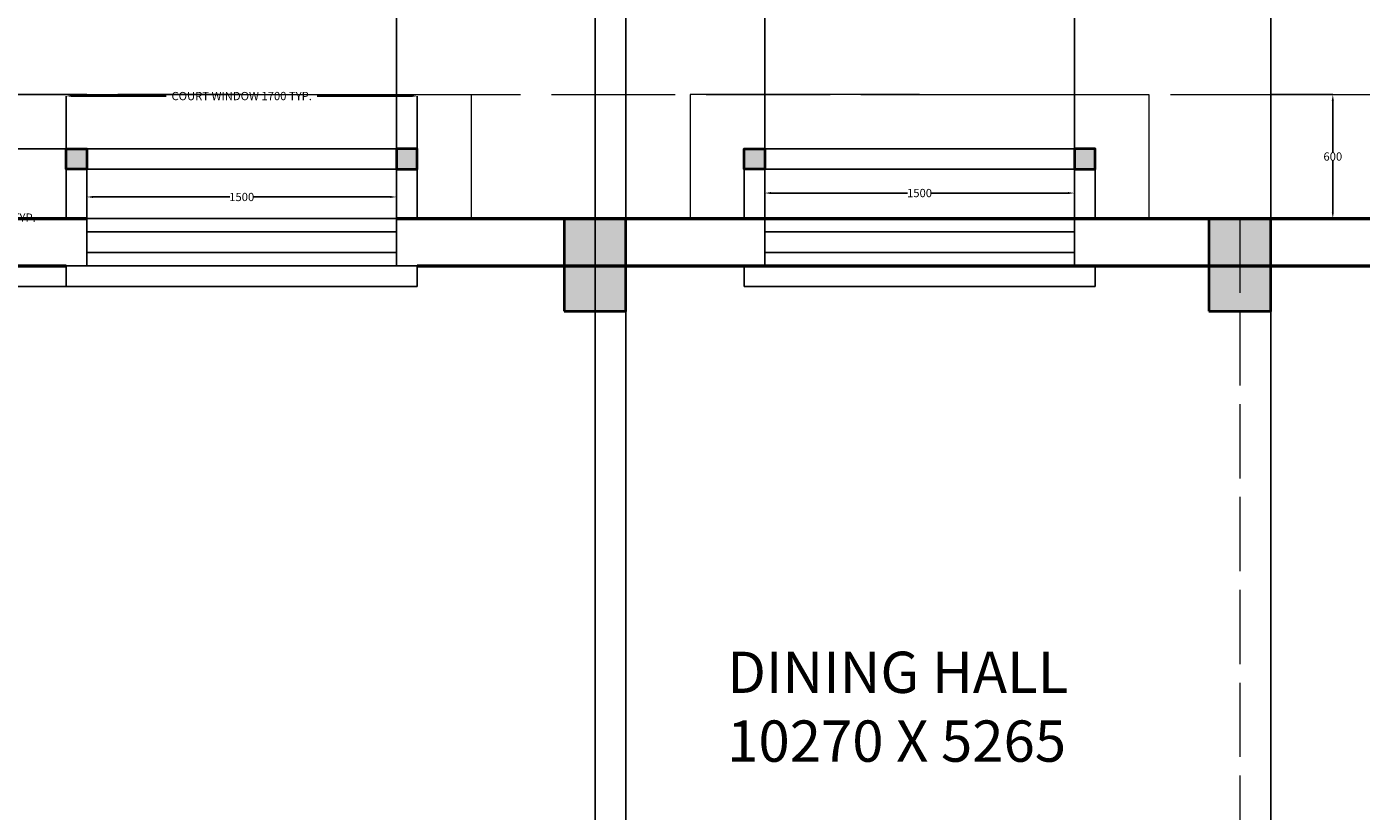
# Model space of a CAD drawing. Units: millimetres. Extents: x -17156 to 39375, y -45872 to -24892.
# Tile 7 of 12: x -5337 to 1128, y -37711 to -33909. Entities that reach past the tile are written whole.
import ezdxf

# ---------------------------------------------------------------- set-up
doc = ezdxf.new("R2010")
doc.units = ezdxf.units.MM
doc.header["$MEASUREMENT"] = 0
doc.linetypes.add('ACAD_ISO02W100', pattern=[15, 12, -3])
for name, color, linetype, lineweight in [('A-ANNO-DIMS', 2, 'Continuous', 18), ('A-AREA-IDEN', 4, 'Continuous', 25), ('A-COLS', 7, 'Continuous', 40), ('A-ROOF', 8, 'Continuous', 18), ('A-ROOF-OVHD', 8, 'ACAD_ISO02W100', 18), ('S-BEAM-OVHD', 8, 'ACAD_ISO02W100', 18), ('WALLS', 5, 'Continuous', 50), ('WINDOW', 240, 'Continuous', 25)]:
    doc.layers.add(name, color=color, linetype=linetype, lineweight=lineweight)
doc.layers.add('A-COLS-PATT', color=114, linetype='Continuous', lineweight=13, true_color=0x139b48)
doc.styles.get("Standard").update_dxf_attribs({"font": 'arial.ttf'})
doc.dimstyles.get("Standard").update_dxf_attribs({"dimtxt": 40, "dimasz": 30.18, "dimexe": 0, "dimexo": 0.0625, "dimgap": 0.09, "dimtad": 0, "dimtih": 1, "dimtoh": 1, "dimdec": 0, "dimzin": 0, "dimdsep": 46, "dimtxsty": 'Standard', "dimcen": 0.09, "dimadec": 0, "dimazin": 0, "dimtfac": 1, "dimtdec": 0, "dimtofl": 0, "dimtmove": 0, "dimatfit": 3, "dimfxl": 1, "dimtolj": 1, "dimtzin": 0, "dimarcsym": 0})

# ---------------------------------------------------------------- blocks, each defined once
blk = doc.blocks.new('*D100')
at = {"layer": 'A-ANNO-DIMS', "color": 0, "lineweight": -2, "transparency": 16777216}
for p, q in [((-5045.8, -34837.8), (-5045.8, -34733.9)), ((-5015.7, -34733.9), (-4353.7, -34733.9)), ((-3576, -34733.9), (-4238, -34733.9)), ((-3545.8, -34837.8), (-3545.8, -34733.9))]:
    blk.add_line(p, q, dxfattribs=at)
at = {"layer": 'A-ANNO-DIMS', "color": 0, "lineweight": 100, "transparency": 16777216}
for points in [[(-5015.7, -34728.9), (-5015.7, -34738.9), (-5045.8, -34733.9)], [(-3576, -34728.9), (-3576, -34738.9), (-3545.8, -34733.9)]]:
    blk.add_solid(points, dxfattribs=at)
at = {"layer": 'Defpoints', "color": 0, "lineweight": 100, "transparency": 16777216}
for p in [(-3545.8, -34733.9), (-5045.8, -34837.8), (-3545.8, -34837.8)]:
    blk.add_point(p, dxfattribs=at)
at = {"layer": 'A-ANNO-DIMS', "color": 0, "transparency": 16777216, "insert": (-4295.8, -34733.9), "char_height": 40, "attachment_point": 5}
blk.add_mtext('\\A1;1500', dxfattribs=at)
blk = doc.blocks.new('*D101')
at = {"layer": 'A-ANNO-DIMS', "color": 0, "lineweight": -2, "transparency": 16777216}
for p, q in [((-1762.3, -34837.8), (-1762.3, -34714.9)), ((-1732.1, -34714.9), (-1070.2, -34714.9)), ((-292.5, -34714.9), (-954.4, -34714.9)), ((-262.3, -34837.8), (-262.3, -34714.9))]:
    blk.add_line(p, q, dxfattribs=at)
at = {"layer": 'A-ANNO-DIMS', "color": 0, "lineweight": 100, "transparency": 16777216}
for points in [[(-1732.1, -34709.8), (-1732.1, -34719.9), (-1762.3, -34714.9)], [(-292.5, -34709.8), (-292.5, -34719.9), (-262.3, -34714.9)]]:
    blk.add_solid(points, dxfattribs=at)
at = {"layer": 'Defpoints', "color": 0, "lineweight": 100, "transparency": 16777216}
for p in [(-262.3, -34714.9), (-1762.3, -34837.8), (-262.3, -34837.8)]:
    blk.add_point(p, dxfattribs=at)
at = {"layer": 'A-ANNO-DIMS', "color": 0, "transparency": 16777216, "insert": (-1012.3, -34714.9), "char_height": 40, "attachment_point": 5}
blk.add_mtext('\\A1;1500', dxfattribs=at)
blk = doc.blocks.new('*D112')
at = {"layer": 'A-ANNO-DIMS', "color": 0, "lineweight": -2, "transparency": 16777216}
for p, q in [((686.4, -34237.8), (989.7, -34237.8)), ((989.7, -34268), (989.7, -34517.3)), ((989.7, -34807.7), (989.7, -34558.4)), ((689.7, -34837.8), (989.7, -34837.8))]:
    blk.add_line(p, q, dxfattribs=at)
at = {"layer": 'A-ANNO-DIMS', "color": 0, "lineweight": 100, "transparency": 16777216}
for points in [[(984.6, -34268), (994.7, -34268), (989.7, -34237.8)], [(984.6, -34807.7), (994.7, -34807.7), (989.7, -34837.8)]]:
    blk.add_solid(points, dxfattribs=at)
at = {"layer": 'Defpoints', "color": 0, "lineweight": 100, "transparency": 16777216}
for p in [(686.3, -34237.8), (689.7, -34837.8), (989.7, -34837.8)]:
    blk.add_point(p, dxfattribs=at)
at = {"layer": 'A-ANNO-DIMS', "color": 0, "transparency": 16777216, "insert": (989.7, -34537.8), "char_height": 40, "attachment_point": 5}
blk.add_mtext('\\A1;600', dxfattribs=at)
blk = doc.blocks.new('WIN-COURTYARD-1500')
for p, q in [((1600, 668), (100, 668)), ((0, 568), (0, 330)), ((100, 568), (100, 330)), ((1600, 568), (100, 568)), ((1600, 568), (1600, 330)), ((1700, 568), (1700, 330)), ((100, 330), (100, 100)), ((100, 330), (1600, 330)), ((1600, 330), (1600, 100)), ((100, 265), (1600, 265)), ((100, 165), (1600, 165)), ((0, 100), (0, 0)), ((0, 100), (100, 100)), ((100, 100), (1700, 100)), ((1700, 0), (1700, 100)), ((0, 0), (1700, 0))]:
    blk.add_line(p, q)
blk = doc.blocks.new('COL-450x300')
h = blk.add_hatch(color=256)
h.dxf.hatch_style = 1
h.paths.add_polyline_path([(0, 300), (0, 0), (450, 0), (450, 300)])
blk.add_lwpolyline([(0, 300), (0, 0), (450, 0), (450, 300)], close=True)
blk = doc.blocks.new('WINDOW-HOOD-2223x600')
for p, q in [((0, 600), (0, 0)), ((1111.5, 600), (0, 600)), ((1111.5, 600), (2223, 600)), ((2223, 600), (2223, 0))]:
    blk.add_line(p, q)
blk = doc.blocks.new('*D140')
at = {"layer": 'A-ANNO-DIMS', "color": 0, "lineweight": -2, "transparency": 16777216}
for p, q in [((-5145.8, -34499.8), (-5145.8, -34244.8)), ((-5115.7, -34244.8), (-4661.6, -34244.8)), ((-3476, -34244.8), (-3930.1, -34244.8)), ((-3445.8, -34499.8), (-3445.8, -34244.8))]:
    blk.add_line(p, q, dxfattribs=at)
at = {"layer": 'A-ANNO-DIMS', "color": 0, "lineweight": 100, "transparency": 16777216}
for points in [[(-5115.7, -34239.8), (-5115.7, -34249.9), (-5145.8, -34244.8)], [(-3476, -34239.8), (-3476, -34249.9), (-3445.8, -34244.8)]]:
    blk.add_solid(points, dxfattribs=at)
at = {"layer": 'Defpoints', "color": 0, "lineweight": 100, "transparency": 16777216}
for p in [(-3445.8, -34244.8), (-5145.8, -34499.8), (-3445.8, -34499.8)]:
    blk.add_point(p, dxfattribs=at)
at = {"layer": 'A-ANNO-DIMS', "color": 0, "transparency": 16777216, "insert": (-4295.8, -34244.8), "char_height": 40, "attachment_point": 5}
blk.add_mtext('\\A1;COURT WINDOW 1700 TYP.', dxfattribs=at)
blk = doc.blocks.new('*D141')
at = {"layer": 'A-ANNO-DIMS', "color": 0, "lineweight": -2, "transparency": 16777216}
for p, q in [((-5145.9, -34499.8), (-5400.8, -34499.8)), ((-5400.8, -34530), (-5400.8, -34813.3)), ((-5400.8, -35137.7), (-5400.8, -34854.4)), ((-5145.9, -35167.8), (-5400.8, -35167.8))]:
    blk.add_line(p, q, dxfattribs=at)
at = {"layer": 'A-ANNO-DIMS', "color": 0, "lineweight": 100, "transparency": 16777216}
for points in [[(-5405.9, -34530), (-5395.8, -34530), (-5400.8, -34499.8)], [(-5405.9, -35137.7), (-5395.8, -35137.7), (-5400.8, -35167.8)]]:
    blk.add_solid(points, dxfattribs=at)
at = {"layer": 'Defpoints', "color": 0, "lineweight": 100, "transparency": 16777216}
for p in [(-5400.8, -34499.8), (-5145.8, -34499.8), (-5145.8, -35167.8)]:
    blk.add_point(p, dxfattribs=at)
at = {"layer": 'A-ANNO-DIMS', "color": 0, "transparency": 16777216, "insert": (-5400.8, -34833.8), "char_height": 40, "attachment_point": 5}
blk.add_mtext('\\A1;668 TYP.', dxfattribs=at)
blk = doc.blocks.new('*D145')
at = {"layer": 'A-ANNO-DIMS', "color": 0, "lineweight": -2, "transparency": 16777216}
for p, q in [((-6237.4, -27247.8), (-17080.3, -27247.8)), ((-17080.3, -27278), (-17080.3, -35684.8)), ((-17080.3, -44132.7), (-17080.3, -35725.9)), ((-2887.4, -44162.8), (-17080.3, -44162.8))]:
    blk.add_line(p, q, dxfattribs=at)
at = {"layer": 'A-ANNO-DIMS', "color": 0, "lineweight": 100, "transparency": 16777216}
for points in [[(-17085.4, -27278), (-17075.3, -27278), (-17080.3, -27247.8)], [(-17085.4, -44132.7), (-17075.3, -44132.7), (-17080.3, -44162.8)]]:
    blk.add_solid(points, dxfattribs=at)
at = {"layer": 'Defpoints', "color": 0, "lineweight": 100, "transparency": 16777216}
for p in [(-6237.3, -27247.8), (-17080.3, -44162.8), (-2887.3, -44162.8)]:
    blk.add_point(p, dxfattribs=at)
at = {"layer": 'A-ANNO-DIMS', "color": 0, "transparency": 16777216, "insert": (-17080.3, -35705.3), "char_height": 40, "attachment_point": 5}
blk.add_mtext('\\A1;16915', dxfattribs=at)
blk = doc.blocks.new('*D148')
at = {"layer": 'A-ANNO-DIMS', "color": 0, "lineweight": -2, "transparency": 16777216}
for p, q in [((-3545.8, -34837.8), (-3545.8, -25564.8)), ((-3515.7, -25564.8), (-2735.5, -25564.8)), ((-1792.5, -25564.8), (-2572.7, -25564.8)), ((-1762.3, -34837.8), (-1762.3, -25564.8))]:
    blk.add_line(p, q, dxfattribs=at)
at = {"layer": 'A-ANNO-DIMS', "color": 0, "lineweight": 100, "transparency": 16777216}
for points in [[(-3515.7, -25559.8), (-3515.7, -25569.9), (-3545.8, -25564.8)], [(-1792.5, -25559.8), (-1792.5, -25569.9), (-1762.3, -25564.8)]]:
    blk.add_solid(points, dxfattribs=at)
at = {"layer": 'Defpoints', "color": 0, "lineweight": 100, "transparency": 16777216}
for p in [(-1762.3, -25564.8), (-3545.8, -34837.8), (-1762.3, -34837.8)]:
    blk.add_point(p, dxfattribs=at)
at = {"layer": 'A-ANNO-DIMS', "color": 0, "transparency": 16777216, "insert": (-2654.1, -25564.8), "char_height": 40, "attachment_point": 5}
blk.add_mtext('\\A1;1783.5', dxfattribs=at)
blk = doc.blocks.new('*D149')
at = {"layer": 'A-ANNO-DIMS', "color": 0, "lineweight": -2, "transparency": 16777216}
for p, q in [((-262.3, -34837.8), (-262.3, -25564.8)), ((-232.1, -25564.8), (601.9, -25564.8)), ((1551.7, -25564.8), (717.6, -25564.8)), ((1581.8, -34837.8), (1581.8, -25564.8))]:
    blk.add_line(p, q, dxfattribs=at)
at = {"layer": 'A-ANNO-DIMS', "color": 0, "lineweight": 100, "transparency": 16777216}
for points in [[(-232.1, -25559.8), (-232.1, -25569.9), (-262.3, -25564.8)], [(1551.7, -25559.8), (1551.7, -25569.9), (1581.8, -25564.8)]]:
    blk.add_solid(points, dxfattribs=at)
at = {"layer": 'Defpoints', "color": 0, "lineweight": 100, "transparency": 16777216}
for p in [(1581.8, -25564.8), (-262.3, -34837.8), (1581.8, -34837.8)]:
    blk.add_point(p, dxfattribs=at)
at = {"layer": 'A-ANNO-DIMS', "color": 0, "transparency": 16777216, "insert": (659.8, -25564.8), "char_height": 40, "attachment_point": 5}
blk.add_mtext('\\A1;1844', dxfattribs=at)
blk = doc.blocks.new('*D151')
at = {"layer": 'A-ANNO-DIMS', "color": 0, "lineweight": -2, "transparency": 16777216}
for p, q in [((-6122.3, -42547.8), (-6122.3, -25564.8)), ((-6092.2, -25564.8), (-4413.2, -25564.8)), ((-2614.5, -25564.8), (-4293.5, -25564.8)), ((-2584.3, -42547.8), (-2584.3, -25564.8))]:
    blk.add_line(p, q, dxfattribs=at)
at = {"layer": 'A-ANNO-DIMS', "color": 0, "lineweight": 100, "transparency": 16777216}
for points in [[(-6092.2, -25559.8), (-6092.2, -25569.9), (-6122.3, -25564.8)], [(-2614.5, -25559.8), (-2614.5, -25569.9), (-2584.3, -25564.8)]]:
    blk.add_solid(points, dxfattribs=at)
at = {"layer": 'Defpoints', "color": 0, "lineweight": 100, "transparency": 16777216}
for p in [(-2584.3, -25564.8), (-6122.3, -42547.8), (-2584.3, -42547.8)]:
    blk.add_point(p, dxfattribs=at)
at = {"layer": 'A-ANNO-DIMS', "color": 0, "transparency": 16777216, "insert": (-4353.3, -25564.8), "char_height": 40, "attachment_point": 5}
blk.add_mtext('\\A1;3538', dxfattribs=at)
blk = doc.blocks.new('*D152')
at = {"layer": 'A-ANNO-DIMS', "color": 0, "lineweight": -2, "transparency": 16777216}
for p, q in [((-2434.3, -40332.8), (-2434.3, -25564.8)), ((-2404.2, -25564.8), (-932.1, -25564.8)), ((659.5, -25564.8), (-812.6, -25564.8)), ((689.7, -40332.8), (689.7, -25564.8))]:
    blk.add_line(p, q, dxfattribs=at)
at = {"layer": 'A-ANNO-DIMS', "color": 0, "lineweight": 100, "transparency": 16777216}
for points in [[(-2404.2, -25559.8), (-2404.2, -25569.9), (-2434.3, -25564.8)], [(659.5, -25559.8), (659.5, -25569.9), (689.7, -25564.8)]]:
    blk.add_solid(points, dxfattribs=at)
at = {"layer": 'Defpoints', "color": 0, "lineweight": 100, "transparency": 16777216}
for p in [(689.7, -25564.8), (-2434.3, -40332.8), (689.7, -40332.8)]:
    blk.add_point(p, dxfattribs=at)
at = {"layer": 'A-ANNO-DIMS', "color": 0, "transparency": 16777216, "insert": (-872.3, -25564.8), "char_height": 40, "attachment_point": 5}
blk.add_mtext('\\A1;3124', dxfattribs=at)

msp = doc.modelspace()

# ---------------------------------------------------------------- hatches: boundary and pattern name
at = {"layer": 'A-COLS-PATT'}
h = msp.add_hatch(color=256, dxfattribs=at)
h.dxf.hatch_style = 1
h.paths.add_polyline_path([(-6007.35, -42547.85, 1), (-6237.35, -42547.85, 1)])
h.paths.add_polyline_path([(-2699.35, -42547.85, 1), (-2469.35, -42547.85, 1)])
h.paths.add_polyline_path([(424.65, -42547.85, 1), (654.65, -42547.85, 1)])
h.paths.add_polyline_path([(3997.65, -42547.85, 1), (4227.65, -42547.85, 1)])
h.paths.add_polyline_path([(1581.84, -34499.85), (1481.84, -34499.85), (1481.84, -34599.85), (1581.84, -34599.85)])
h.paths.add_polyline_path([(3181.84, -34499.85), (3081.84, -34499.85), (3081.84, -34599.85), (3181.84, -34599.85)])
h.paths.add_polyline_path([(-162.32, -34499.85), (-262.32, -34499.85), (-262.32, -34599.85), (-162.32, -34599.85)])
h.paths.add_polyline_path([(-1762.32, -34499.85), (-1862.32, -34499.85), (-1862.32, -34599.85), (-1762.32, -34599.85)])
h.paths.add_polyline_path([(-3445.85, -34499.85), (-3545.85, -34499.85), (-3545.85, -34599.85), (-3445.85, -34599.85)])
h.paths.add_polyline_path([(-5045.85, -34499.85), (-5145.85, -34499.85), (-5145.85, -34599.85), (-5045.85, -34599.85)])

# ---------------------------------------------------------------- linework, layer by layer
at = {"layer": 'A-COLS'}
for points in [[(-5045.85, -34599.85), (-5145.85, -34599.85), (-5145.85, -34499.85), (-5045.85, -34499.85)], [(-3545.85, -34599.85), (-3445.85, -34599.85), (-3445.85, -34499.85), (-3545.85, -34499.85)], [(-1762.32, -34599.85), (-1862.32, -34599.85), (-1862.32, -34499.85), (-1762.32, -34499.85)], [(-262.32, -34599.85), (-162.32, -34599.85), (-162.32, -34499.85), (-262.32, -34499.85)]]:
    msp.add_lwpolyline(points, close=True, dxfattribs=at)
at = {"layer": 'A-ROOF'}
msp.add_line((-5407.35, -34237.85), (-3184.35, -34237.85), dxfattribs=at)
at = {"layer": 'A-ROOF-OVHD', "ltscale": 50}
for p, q in [((-4295.85, -34237.85), (-5407.35, -34237.85)), ((-4295.85, -34237.85), (-3184.35, -34237.85)), ((-3545.85, -34237.85), (3662.65, -34237.85)), ((-3184.35, -34237.85), (-3184.35, -34837.85))]:
    msp.add_line(p, q, dxfattribs=at)
at = {"layer": 'S-BEAM-OVHD', "ltscale": 30}
for p, q in [((-2584.35, -34837.85), (-2584.35, -40782.85)), ((539.65, -34837.85), (539.65, -40782.85))]:
    msp.add_line(p, q, dxfattribs=at)
at = {"layer": 'WALLS'}
for p, q in [((-8859.1, -34837.85), (-5045.85, -34837.85)), ((-3545.85, -34837.85), (4262.65, -34837.85)), ((-8852.35, -35067.85), (-5145.85, -35067.85)), ((-3445.85, -35067.85), (4262.65, -35067.85))]:
    msp.add_line(p, q, dxfattribs=at)

# ---------------------------------------------------------------- block references
at = {"layer": 'A-COLS'}
for p, rotation in [((-2434.35, -35287.85), 90.00000000000134), ((689.65, -35287.85), 90.00000000000124)]:
    msp.add_blockref('COL-450x300', p, dxfattribs=dict(at, rotation=rotation))
at = {"layer": 'A-ROOF'}
msp.add_blockref('WINDOW-HOOD-2223x600', (-2123.82, -34837.85), dxfattribs=at)
at = {"layer": 'WINDOW'}
for p in [(-5145.85, -35167.85), (-1862.32, -35167.85)]:
    msp.add_blockref('WIN-COURTYARD-1500', p, dxfattribs=at)

# ---------------------------------------------------------------- texts
at = {"layer": 'A-AREA-IDEN', "insert": (-1943.96, -36937.6), "char_height": 200, "attachment_point": 1}
msp.add_mtext_dynamic_manual_height_columns('{DINING HALL\\P10270 X 5265}', width=1770.4181, gutter_width=1, heights=[0], dxfattribs=at)

# ---------------------------------------------------------------- dimensions: what is measured, and where the dimension line sits
at = {"layer": 'A-ANNO-DIMS'}
for base, p1, p2, override, picture, middle in [((-2584.35, -25564.85), (-6122.35, -42547.85), (-2584.35, -42547.85), {"dimdec": 0, "dimlfac": 1, "dimrnd": 0, "dimzin": 0, "dimdsep": 46, "dimlunit": 2}, '*D151', (-4353.35, -25564.85)), ((-1762.32, -25564.85), (-3545.85, -34837.85), (-1762.32, -34837.85), {"dimdec": 1, "dimlfac": 1, "dimrnd": 0, "dimzin": 0, "dimdsep": 46, "dimlunit": 2}, '*D148', (-2654.08, -25564.85)), ((689.65, -25564.85), (-2434.35, -40332.85), (689.65, -40332.85), {"dimdec": 0, "dimlfac": 1, "dimrnd": 0, "dimzin": 0, "dimdsep": 46, "dimlunit": 2}, '*D152', (-872.35, -25564.85)), ((1581.84, -25564.85), (-262.32, -34837.85), (1581.84, -34837.85), {"dimdec": 0, "dimlfac": 1, "dimrnd": 0, "dimzin": 0, "dimdsep": 46, "dimlunit": 2}, '*D149', (659.76, -25564.85)), ((-3545.85, -34733.91), (-5045.85, -34837.85), (-3545.85, -34837.85), {"dimclrd": 0, "dimclre": 0, "dimclrt": 0}, '*D100', (-4295.85, -34733.91)), ((-262.32, -34714.85), (-1762.32, -34837.85), (-262.32, -34837.85), {"dimclrd": 0, "dimclre": 0, "dimclrt": 0}, '*D101', (-1012.32, -34714.85))]:
    dim = msp.add_linear_dim(base=base, p1=p1, p2=p2, dimstyle='Standard', override=override, dxfattribs=at)
    dim.commit()
    dim.dimension.update_dxf_attribs({"geometry": picture, "text_midpoint": middle})
for base, p1, p2, override, picture, middle in [((-17080.35, -44162.85), (-6237.35, -27247.85), (-2887.35, -44162.85), {"dimdec": 0, "dimlfac": 1, "dimrnd": 0, "dimzin": 0, "dimdsep": 46, "dimlunit": 2}, '*D145', (-17080.35, -35705.35)), ((989.65, -34837.85), (686.3, -34237.85), (689.65, -34837.85), {"dimclrd": 0, "dimclre": 0, "dimclrt": 0}, '*D112', (989.65, -34537.85))]:
    dim = msp.add_linear_dim(base=base, p1=p1, p2=p2, angle=90, dimstyle='Standard', override=override, dxfattribs=at)
    dim.commit()
    dim.dimension.update_dxf_attribs({"geometry": picture, "text_midpoint": middle})
dim = msp.add_linear_dim(base=(-3445.85, -34244.85), p1=(-5145.85, -34499.85), p2=(-3445.85, -34499.85), text='COURT WINDOW <> TYP.', dimstyle='Standard', override={"dimdec": 0, "dimlfac": 1, "dimrnd": 0, "dimzin": 0, "dimdsep": 46, "dimlunit": 2}, dxfattribs=at)
dim.commit()
dim.dimension.update_dxf_attribs({"geometry": '*D140', "text_midpoint": (-4295.85, -34244.85)})
dim = msp.add_linear_dim(base=(-5400.85, -34499.85), p1=(-5145.85, -35167.85), p2=(-5145.85, -34499.85), angle=90, text='<> TYP.', dimstyle='Standard', override={"dimdec": 0, "dimlfac": 1, "dimrnd": 0, "dimzin": 0, "dimdsep": 46, "dimlunit": 2}, dxfattribs=at)
dim.commit()
dim.dimension.update_dxf_attribs({"geometry": '*D141', "text_midpoint": (-5400.85, -34833.85)})

doc.saveas('drawing.dxf')
